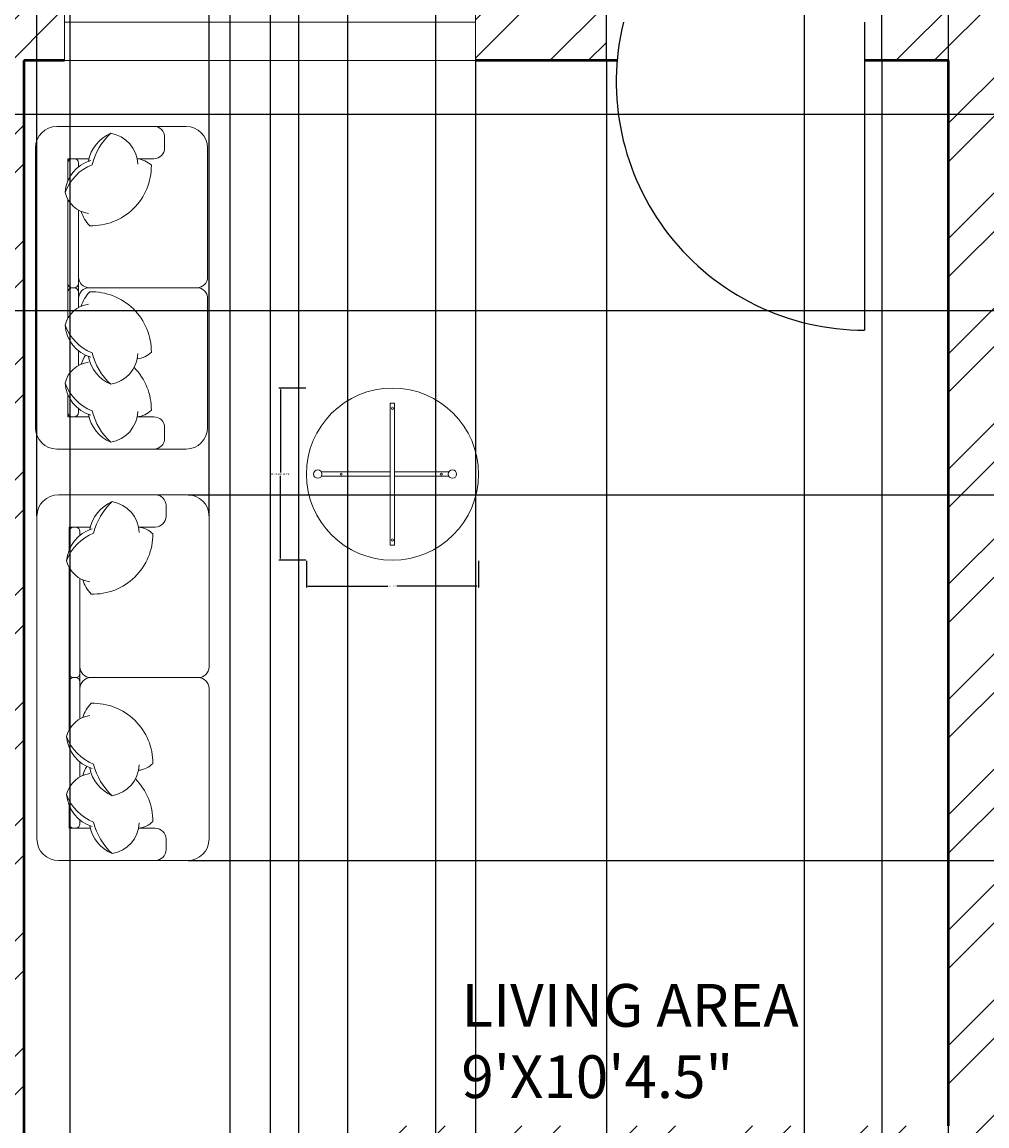
# Model space of a CAD drawing. Units: inches. Extents: x 1980 to 2738, y 1471 to 2568.
# Tile 9 of 22: x 2250 to 2363, y 1878 to 2007. Entities that reach past the tile are written whole.
import ezdxf

# ---------------------------------------------------------------- set-up
doc = ezdxf.new("R2010")
doc.units = ezdxf.units.IN
for name, color, linetype, lineweight in [('A-ANNO-DIMS', 2, 'Continuous', 18), ('A-AREA-IDEN', 7, 'Continuous', 18), ('A-DOOR', 31, 'Continuous', 25), ('A-FURN', 8, 'Continuous', 18), ('A-GLAZ', 141, 'Continuous', 18), ('A-WALL', 7, 'Continuous', 50)]:
    doc.layers.add(name, color=color, linetype=linetype, lineweight=lineweight)
doc.layers.add('A-WALL-PATT', color=9, linetype='Continuous', lineweight=13, true_color=0xd19cc7)
doc.styles.get("Standard").update_dxf_attribs({"font": 'arial.ttf'})
doc.dimstyles.get("Standard").update_dxf_attribs({"dimtxt": 0.18, "dimasz": 0.18, "dimexe": 0.18, "dimexo": 0.0625, "dimgap": 0.09, "dimtad": 0, "dimtih": 1, "dimtoh": 1, "dimdec": 4, "dimzin": 0, "dimdsep": 46, "dimtxsty": 'Standard', "dimcen": 0.09, "dimadec": 0, "dimazin": 0, "dimtfac": 1, "dimtdec": 4, "dimtofl": 0, "dimtmove": 0, "dimatfit": 3, "dimfxl": 1, "dimtolj": 1, "dimtzin": 0, "dimarcsym": 0})

# ---------------------------------------------------------------- blocks, each defined once
blk = doc.blocks.new('table r 343')
at = {"color": 0}
for p, q in [((-10, 10), (-10, 262.1)), ((10, 10), (10, 262.1)), ((-330.3, 10), (330.3, 10)), ((-330.3, 10), (-330.3, -10)), ((330.3, 10), (330.3, -10)), ((-330.3, -10), (330.3, -10)), ((-10, -330.3), (-10, -10)), ((10, -330.3), (10, -10))]:
    blk.add_line(p, q, dxfattribs=at)
for centre, radius in [((0, 0), 400), ((0, 278.7), 19.4), ((0, 226.8), 5), ((-306.1, 0), 5), ((306.1, 0), 5), ((0, -238.1), 5), ((0, -346.9), 19.4)]:
    blk.add_circle(centre, radius, dxfattribs=at)
blk = doc.blocks.new('WIN-48IN-WALL')
for p, q in [((0, 4.5), (0, 9)), ((0, 9), (0, 0)), ((48, 9), (0, 9)), ((48, 0), (48, 9)), ((48, 9), (48, 4.5)), ((48, 4.5), (0, 4.5)), ((0, 0), (48, 0))]:
    blk.add_line(p, q)
blk = doc.blocks.new('*D19')
at = {"layer": 'A-ANNO-DIMS', "color": 0, "lineweight": -2, "transparency": 16777216}
for p, q in [((2283.52, 1963.93), (2280.38, 1963.93)), ((2280.56, 1963.75), (2280.56, 1954.06)), ((2280.56, 1944), (2280.56, 1953.69)), ((2283.52, 1943.82), (2280.38, 1943.82))]:
    blk.add_line(p, q, dxfattribs=at)
at = {"layer": 'A-ANNO-DIMS', "color": 0, "transparency": 16777216}
for points in [[(2280.53, 1963.75), (2280.59, 1963.75), (2280.56, 1963.93)], [(2280.53, 1944), (2280.59, 1944), (2280.56, 1943.82)]]:
    blk.add_solid(points, dxfattribs=at)
at = {"layer": 'Defpoints', "color": 0, "transparency": 16777216}
for p in [(2283.58, 1963.93), (2280.56, 1943.82), (2283.58, 1943.82)]:
    blk.add_point(p, dxfattribs=at)
at = {"layer": 'A-ANNO-DIMS', "color": 0, "transparency": 16777216, "insert": (2280.56, 1953.88), "char_height": 0.18, "attachment_point": 5}
blk.add_mtext('\\A1;END TABLE 20 TYP.', dxfattribs=at)
blk = doc.blocks.new('*D20')
at = {"layer": 'A-ANNO-DIMS', "color": 0, "lineweight": -2, "transparency": 16777216}
for p, q in [((2283.58, 1943.76), (2283.58, 1940.62)), ((2303.69, 1943.76), (2303.69, 1940.62)), ((2283.76, 1940.8), (2293.1, 1940.8)), ((2303.51, 1940.8), (2294.16, 1940.8))]:
    blk.add_line(p, q, dxfattribs=at)
at = {"layer": 'A-ANNO-DIMS', "color": 0, "transparency": 16777216}
for points in [[(2283.76, 1940.83), (2283.76, 1940.77), (2283.58, 1940.8)], [(2303.51, 1940.83), (2303.51, 1940.77), (2303.69, 1940.8)]]:
    blk.add_solid(points, dxfattribs=at)
at = {"layer": 'Defpoints', "color": 0, "transparency": 16777216}
for p in [(2283.58, 1943.82), (2303.69, 1943.82), (2303.69, 1940.8)]:
    blk.add_point(p, dxfattribs=at)
at = {"layer": 'A-ANNO-DIMS', "color": 0, "transparency": 16777216, "insert": (2293.63, 1940.8), "char_height": 0.18, "attachment_point": 5}
blk.add_mtext('\\A1;20 TYP.', dxfattribs=at)
blk = doc.blocks.new('*D40')
at = {"layer": 'A-ANNO-DIMS', "color": 0, "lineweight": -2, "transparency": 16777216}
for p, q in [((2218.65, 2053.14), (2218.65, 1533.71)), ((2298.65, 2053.14), (2298.65, 1533.71)), ((2218.83, 1533.89), (2258.43, 1533.89)), ((2298.47, 1533.89), (2258.87, 1533.89))]:
    blk.add_line(p, q, dxfattribs=at)
at = {"layer": 'A-ANNO-DIMS', "color": 0, "transparency": 16777216}
for points in [[(2218.83, 1533.92), (2218.83, 1533.86), (2218.65, 1533.89)], [(2298.47, 1533.92), (2298.47, 1533.86), (2298.65, 1533.89)]]:
    blk.add_solid(points, dxfattribs=at)
at = {"layer": 'Defpoints', "color": 0, "transparency": 16777216}
for p in [(2218.65, 2053.21), (2298.65, 2053.21), (2298.65, 1533.89)]:
    blk.add_point(p, dxfattribs=at)
at = {"layer": 'A-ANNO-DIMS', "color": 0, "transparency": 16777216, "insert": (2258.65, 1533.89), "char_height": 0.18, "attachment_point": 5}
blk.add_mtext('\\A1;80', dxfattribs=at)
blk = doc.blocks.new('*D41')
at = {"layer": 'A-ANNO-DIMS', "color": 0, "lineweight": -2, "transparency": 16777216}
for p, q in [((2298.65, 2095.14), (2298.65, 1533.71)), ((2515.4, 2095.14), (2515.4, 1533.71)), ((2298.83, 1533.89), (2406.56, 1533.89)), ((2515.22, 1533.89), (2407.49, 1533.89))]:
    blk.add_line(p, q, dxfattribs=at)
at = {"layer": 'A-ANNO-DIMS', "color": 0, "transparency": 16777216}
for points in [[(2298.83, 1533.92), (2298.83, 1533.86), (2298.65, 1533.89)], [(2515.22, 1533.92), (2515.22, 1533.86), (2515.4, 1533.89)]]:
    blk.add_solid(points, dxfattribs=at)
at = {"layer": 'Defpoints', "color": 0, "transparency": 16777216}
for p in [(2298.65, 2095.21), (2515.4, 2095.21), (2515.4, 1533.89)]:
    blk.add_point(p, dxfattribs=at)
at = {"layer": 'A-ANNO-DIMS', "color": 0, "transparency": 16777216, "insert": (2407.03, 1533.89), "char_height": 0.18, "attachment_point": 5}
blk.add_mtext('\\A1;216.75', dxfattribs=at)
blk = doc.blocks.new('*D45')
at = {"layer": 'A-ANNO-DIMS', "color": 0, "lineweight": -2, "transparency": 16777216}
for p, q in [((2255.99, 1694.77), (2255.99, 2507.54)), ((2256.17, 2507.36), (2267.22, 2507.36)), ((2279.21, 2507.36), (2268.15, 2507.36)), ((2279.39, 1694.77), (2279.39, 2507.54))]:
    blk.add_line(p, q, dxfattribs=at)
at = {"layer": 'A-ANNO-DIMS', "color": 0, "transparency": 16777216}
for points in [[(2256.17, 2507.39), (2256.17, 2507.33), (2255.99, 2507.36)], [(2279.21, 2507.39), (2279.21, 2507.33), (2279.39, 2507.36)]]:
    blk.add_solid(points, dxfattribs=at)
at = {"layer": 'Defpoints', "color": 0, "transparency": 16777216}
for p in [(2279.39, 2507.36), (2255.99, 1694.71), (2279.39, 1694.71)]:
    blk.add_point(p, dxfattribs=at)
at = {"layer": 'A-ANNO-DIMS', "color": 0, "transparency": 16777216, "insert": (2267.69, 2507.36), "char_height": 0.18, "attachment_point": 5}
blk.add_mtext('\\A1;23.407', dxfattribs=at)
blk = doc.blocks.new('*D50')
at = {"layer": 'A-ANNO-DIMS', "color": 0, "lineweight": -2, "transparency": 16777216}
for p, q in [((2288.43, 1708.09), (2288.43, 2507.54)), ((2288.61, 2507.36), (2314.71, 2507.36)), ((2341.6, 2507.36), (2315.5, 2507.36)), ((2341.78, 1708.09), (2341.78, 2507.54))]:
    blk.add_line(p, q, dxfattribs=at)
at = {"layer": 'A-ANNO-DIMS', "color": 0, "transparency": 16777216}
for points in [[(2288.61, 2507.39), (2288.61, 2507.33), (2288.43, 2507.36)], [(2341.6, 2507.39), (2341.6, 2507.33), (2341.78, 2507.36)]]:
    blk.add_solid(points, dxfattribs=at)
at = {"layer": 'Defpoints', "color": 0, "transparency": 16777216}
for p in [(2341.78, 2507.36), (2288.43, 1708.03), (2341.78, 1708.03)]:
    blk.add_point(p, dxfattribs=at)
at = {"layer": 'A-ANNO-DIMS', "color": 0, "transparency": 16777216, "insert": (2315.11, 2507.36), "char_height": 0.18, "attachment_point": 5}
blk.add_mtext('\\A1;53.34', dxfattribs=at)
blk = doc.blocks.new('*D51')
at = {"layer": 'A-ANNO-DIMS', "color": 0, "lineweight": -2, "transparency": 16777216}
for p, q in [((2341.78, 1708.09), (2341.78, 2507.54)), ((2341.96, 2507.36), (2349.72, 2507.36)), ((2358.4, 2507.36), (2350.63, 2507.36)), ((2358.58, 1694.77), (2358.58, 2507.54))]:
    blk.add_line(p, q, dxfattribs=at)
at = {"layer": 'A-ANNO-DIMS', "color": 0, "transparency": 16777216}
for points in [[(2341.96, 2507.39), (2341.96, 2507.33), (2341.78, 2507.36)], [(2358.4, 2507.39), (2358.4, 2507.33), (2358.58, 2507.36)]]:
    blk.add_solid(points, dxfattribs=at)
at = {"layer": 'Defpoints', "color": 0, "transparency": 16777216}
for p in [(2358.58, 2507.36), (2341.78, 1708.03), (2358.58, 1694.71)]:
    blk.add_point(p, dxfattribs=at)
at = {"layer": 'A-ANNO-DIMS', "color": 0, "transparency": 16777216, "insert": (2350.18, 2507.36), "char_height": 0.18, "attachment_point": 5}
blk.add_mtext('\\A1;16.807', dxfattribs=at)
blk = doc.blocks.new('*D53')
at = {"layer": 'A-ANNO-DIMS', "color": 0, "lineweight": -2, "transparency": 16777216}
for p, q in [((2318.63, 2002.14), (2318.63, 1533.71)), ((2350.79, 2002.14), (2350.79, 1533.71)), ((2318.81, 1533.89), (2334.25, 1533.89)), ((2350.61, 1533.89), (2335.18, 1533.89))]:
    blk.add_line(p, q, dxfattribs=at)
at = {"layer": 'A-ANNO-DIMS', "color": 0, "transparency": 16777216}
for points in [[(2318.81, 1533.92), (2318.81, 1533.86), (2318.63, 1533.89)], [(2350.61, 1533.92), (2350.61, 1533.86), (2350.79, 1533.89)]]:
    blk.add_solid(points, dxfattribs=at)
at = {"layer": 'Defpoints', "color": 0, "transparency": 16777216}
for p in [(2318.63, 2002.21), (2350.79, 2002.21), (2350.79, 1533.89)]:
    blk.add_point(p, dxfattribs=at)
at = {"layer": 'A-ANNO-DIMS', "color": 0, "transparency": 16777216, "insert": (2334.71, 1533.89), "char_height": 0.18, "attachment_point": 5}
blk.add_mtext('\\A1;32.155', dxfattribs=at)
blk = doc.blocks.new('*D54')
at = {"layer": 'A-ANNO-DIMS', "color": 0, "lineweight": -2, "transparency": 16777216}
for p, q in [((2252.1, 1949.01), (2252.1, 2507.54)), ((2252.28, 2507.36), (2261.78, 2507.36)), ((2272.03, 2507.36), (2262.53, 2507.36)), ((2272.21, 1949.01), (2272.21, 2507.54))]:
    blk.add_line(p, q, dxfattribs=at)
at = {"layer": 'A-ANNO-DIMS', "color": 0, "transparency": 16777216}
for points in [[(2252.28, 2507.39), (2252.28, 2507.33), (2252.1, 2507.36)], [(2272.03, 2507.39), (2272.03, 2507.33), (2272.21, 2507.36)]]:
    blk.add_solid(points, dxfattribs=at)
at = {"layer": 'Defpoints', "color": 0, "transparency": 16777216}
for p in [(2272.21, 2507.36), (2252.1, 1948.95), (2272.21, 1948.95)]:
    blk.add_point(p, dxfattribs=at)
at = {"layer": 'A-ANNO-DIMS', "color": 0, "transparency": 16777216, "insert": (2262.16, 2507.36), "char_height": 0.18, "attachment_point": 5}
blk.add_mtext('\\A1;20.11', dxfattribs=at)
blk = doc.blocks.new('*D55')
at = {"layer": 'A-ANNO-DIMS', "color": 0, "lineweight": -2, "transparency": 16777216}
for p, q in [((2269.76, 1951.46), (2689.91, 1951.46)), ((2689.73, 1951.28), (2689.73, 1930.28)), ((2689.73, 1908.91), (2689.73, 1929.91)), ((2269.76, 1908.73), (2689.91, 1908.73))]:
    blk.add_line(p, q, dxfattribs=at)
at = {"layer": 'A-ANNO-DIMS', "color": 0, "transparency": 16777216}
for points in [[(2689.7, 1951.28), (2689.76, 1951.28), (2689.73, 1951.46)], [(2689.7, 1908.91), (2689.76, 1908.91), (2689.73, 1908.73)]]:
    blk.add_solid(points, dxfattribs=at)
at = {"layer": 'Defpoints', "color": 0, "transparency": 16777216}
for p in [(2269.7, 1951.46), (2689.73, 1951.46), (2269.7, 1908.73)]:
    blk.add_point(p, dxfattribs=at)
at = {"layer": 'A-ANNO-DIMS', "color": 0, "transparency": 16777216, "insert": (2689.73, 1930.09), "char_height": 0.18, "attachment_point": 5}
blk.add_mtext('\\A1;42.735', dxfattribs=at)
blk = doc.blocks.new('*D56')
at = {"layer": 'A-ANNO-DIMS', "color": 0, "lineweight": -2, "transparency": 16777216}
for p, q in [((2114.15, 1995.93), (2689.91, 1995.93)), ((2689.73, 1995.75), (2689.73, 1984.65)), ((2689.73, 1973.18), (2689.73, 1984.28)), ((2114.15, 1973), (2689.91, 1973))]:
    blk.add_line(p, q, dxfattribs=at)
at = {"layer": 'A-ANNO-DIMS', "color": 0, "transparency": 16777216}
for points in [[(2689.7, 1995.75), (2689.76, 1995.75), (2689.73, 1995.93)], [(2689.7, 1973.18), (2689.76, 1973.18), (2689.73, 1973)]]:
    blk.add_solid(points, dxfattribs=at)
at = {"layer": 'Defpoints', "color": 0, "transparency": 16777216}
for p in [(2114.08, 1995.93), (2689.73, 1995.93), (2114.08, 1973)]:
    blk.add_point(p, dxfattribs=at)
at = {"layer": 'A-ANNO-DIMS', "color": 0, "transparency": 16777216, "insert": (2689.73, 1984.47), "char_height": 0.18, "attachment_point": 5}
blk.add_mtext('\\A1;22.935', dxfattribs=at)
blk = doc.blocks.new('*D64')
at = {"layer": 'A-ANNO-DIMS', "color": 0, "lineweight": -2, "transparency": 16777216}
for p, q in [((2303.33, 2002.14), (2303.33, 1533.71)), ((2318.63, 2002.14), (2318.63, 1533.71)), ((2303.51, 1533.89), (2310.67, 1533.89)), ((2318.45, 1533.89), (2311.3, 1533.89))]:
    blk.add_line(p, q, dxfattribs=at)
at = {"layer": 'A-ANNO-DIMS', "color": 0, "transparency": 16777216}
for points in [[(2303.51, 1533.92), (2303.51, 1533.86), (2303.33, 1533.89)], [(2318.45, 1533.92), (2318.45, 1533.86), (2318.63, 1533.89)]]:
    blk.add_solid(points, dxfattribs=at)
at = {"layer": 'Defpoints', "color": 0, "transparency": 16777216}
for p in [(2303.33, 2002.21), (2318.63, 2002.21), (2318.63, 1533.89)]:
    blk.add_point(p, dxfattribs=at)
at = {"layer": 'A-ANNO-DIMS', "color": 0, "transparency": 16777216, "insert": (2310.98, 1533.89), "char_height": 0.18, "attachment_point": 5}
blk.add_mtext('\\A1;15.3', dxfattribs=at)
blk = doc.blocks.new('*D66')
at = {"layer": 'A-ANNO-DIMS', "color": 0, "lineweight": -2, "transparency": 16777216}
for p, q in [((2274.65, 2095.14), (2274.65, 1533.71)), ((2282.65, 2095.14), (2282.65, 1533.71)), ((2274.83, 1533.89), (2278.5, 1533.89)), ((2282.47, 1533.89), (2278.8, 1533.89))]:
    blk.add_line(p, q, dxfattribs=at)
at = {"layer": 'A-ANNO-DIMS', "color": 0, "transparency": 16777216}
for points in [[(2274.83, 1533.92), (2274.83, 1533.86), (2274.65, 1533.89)], [(2282.47, 1533.92), (2282.47, 1533.86), (2282.65, 1533.89)]]:
    blk.add_solid(points, dxfattribs=at)
at = {"layer": 'Defpoints', "color": 0, "transparency": 16777216}
for p in [(2274.65, 2095.21), (2282.65, 2095.21), (2282.65, 1533.89)]:
    blk.add_point(p, dxfattribs=at)
at = {"layer": 'A-ANNO-DIMS', "color": 0, "transparency": 16777216, "insert": (2278.65, 1533.89), "char_height": 0.18, "attachment_point": 5}
blk.add_mtext('\\A1;8', dxfattribs=at)

msp = doc.modelspace()

# ---------------------------------------------------------------- hatches: boundary and pattern name
at = {"layer": 'A-WALL-PATT'}
h = msp.add_hatch(dxfattribs=at)
h.set_pattern_fill('ANSI32', color=256)
h.paths.add_polyline_path([(2257.5661, 2416.2064), (2257.5661, 2420.7064), (2250.5833, 2420.7064), (2250.5833, 2462.7064), (2246.0833, 2462.7064), (2246.0833, 2420.7064), (2237.0791, 2420.7064), (2237.0791, 2411.7064), (2246.0833, 2411.7064), (2246.0833, 2291.7064), (2242.6109, 2291.7064), (2242.6109, 2287.2064), (2246.0833, 2287.2064), (2250.5833, 2287.2064), (2250.5833, 2291.7064), (2250.5833, 2411.7064), (2257.5661, 2411.7064)])
h.paths.add_polyline_path([(2387.0396, 2416.2064), (2387.0396, 2420.7064), (2367.5833, 2420.7064), (2367.5833, 2462.7064), (2358.5833, 2462.7064), (2358.5833, 2420.7064), (2329.3087, 2420.7064), (2329.3087, 2411.7064), (2358.5833, 2411.7064), (2358.5833, 2321.7275), (2358.5833, 2309.7064), (2347.3089, 2309.7064), (2293.3089, 2309.7064), (2293.3089, 2259.0771), (2297.8089, 2259.0771), (2297.8089, 2305.2064), (2347.3089, 2305.2064), (2347.3089, 2284.7412), (2351.8089, 2284.7412), (2351.8089, 2305.2064), (2372.3188, 2305.2064), (2372.3761, 2284.3899), (2377.0295, 2284.3899), (2377.0295, 2299.3058), (2377.0295, 2305.2064), (2426.5295, 2305.2064), (2426.5295, 2257.5573), (2431.0295, 2257.5573), (2431.0295, 2309.7064), (2377.0295, 2309.7064), (2367.5833, 2309.7064), (2367.5833, 2321.7275), (2367.5833, 2411.7064), (2387.0396, 2411.7064)])
h.paths.add_polyline_path([(2448.5267, 2416.2064), (2448.5267, 2420.7064), (2423.0396, 2420.7064), (2423.0396, 2411.7064), (2448.5267, 2411.7064)])
h.paths.add_polyline_path([(2130.9128, 2416.2064), (2130.9128, 2420.7064), (2105.0833, 2420.7064), (2105.0833, 2386.6942), (2114.0833, 2386.6942), (2114.0833, 2411.7064), (2130.9128, 2411.7064)])
h.paths.add_polyline_path([(2212.9478, 2420.7064), (2190.9128, 2420.7064), (2190.9128, 2411.7064), (2212.9478, 2411.7064), (2212.9478, 2416.2064)])
h.paths.add_polyline_path([(2114.0833, 2326.6942), (2105.0833, 2326.6942), (2105.0833, 2291.7064), (2081.0833, 2291.7064), (2081.0833, 2287.2064), (2105.0833, 2287.2064), (2105.0833, 2276.1935), (2114.0833, 2276.1935), (2114.0833, 2287.2064), (2166.3825, 2287.2064), (2166.3825, 2289.4564), (2166.3825, 2291.7064), (2114.0833, 2291.7064)])
h.paths.add_polyline_path([(2114.0833, 2252.1935), (2105.0833, 2252.1935), (2105.0833, 2233.2064), (2081.0833, 2233.2064), (2081.0833, 2228.7064), (2105.0833, 2228.7064), (2105.0833, 2213.4478), (2114.0833, 2213.4478), (2114.0833, 2228.7064), (2195.0833, 2228.7064), (2199.5833, 2228.7064), (2208.4455, 2228.7064), (2208.4455, 2230.9564), (2208.4455, 2233.2064), (2199.5833, 2233.2064), (2199.5833, 2287.2064), (2206.8904, 2287.2064), (2206.8904, 2289.4564), (2206.8904, 2291.7064), (2189.446, 2291.7064), (2189.446, 2289.4564), (2189.446, 2287.2064), (2195.0833, 2287.2064), (2195.0833, 2233.2064), (2114.0833, 2233.2064)])
h.paths.add_polyline_path([(2114.0833, 2153.4478), (2109.5833, 2153.4478), (2105.0833, 2153.4478), (2105.0833, 2135.2374), (2114.0833, 2135.2374)], flags=17)
h.paths.add_polyline_path([(2135.9619, 2095.4081), (2140.1805, 2095.4081), (2140.1805, 2104.2064), (2114.0833, 2104.2064), (2114.0833, 2110.3997), (2109.5833, 2110.3997), (2105.0833, 2110.3997), (2105.0833, 2104.2064), (2081.0833, 2104.2064), (2081.0833, 2099.7064), (2105.0833, 2099.7064), (2127.5416, 2099.8532), (2127.5416, 2056.9393), (2136.2133, 2056.9393)], flags=17)
h.paths.add_polyline_path([(2255.4895, 2104.2064), (2250.5833, 2104.2064), (2250.5833, 2233.2064), (2246.0833, 2233.2064), (2242.4941, 2233.2064), (2242.4941, 2228.7064), (2246.0833, 2228.7064), (2246.0833, 2104.2064), (2163.6825, 2104.2064), (2163.6825, 2099.8072), (2163.6825, 2095.4081), (2191.4325, 2095.4081), (2191.4325, 2011.2064), (2186.0833, 2011.2064), (2136.5143, 2010.8824), (2136.3702, 2032.9403), (2131.9559, 2032.9115), (2127.5416, 2032.8826), (2127.5416, 2006.7064), (2105.0833, 2006.7064), (2081.0833, 2006.7064), (2081.0833, 2002.2064), (2105.0833, 2002.2064), (2105.0833, 1995.9329), (2114.0833, 1995.9329), (2114.0833, 2002.2064), (2246.0833, 2002.2064), (2246.0833, 1877.7064), (2242.1358, 1877.7064), (2242.1358, 1873.2064), (2250.5833, 1873.2064), (2250.5833, 2002.2064), (2255.3335, 2002.2064), (2255.3335, 2011.2064), (2195.9325, 2011.2064), (2195.9325, 2095.2064), (2255.4895, 2095.2064), (2255.4895, 2099.5471)])
h.paths.add_polyline_path([(2199.5833, 1873.2064), (2209.827, 1873.2064), (2209.827, 1875.4564), (2209.827, 1877.7064), (2114.0833, 1877.7064), (2114.0833, 1890.0968), (2105.0833, 1890.0968), (2105.0833, 1877.7064), (2081.0833, 1877.7064), (2081.0833, 1873.2064), (2105.0833, 1873.2064), (2105.0833, 1857.7279), (2114.0833, 1857.7279), (2114.0833, 1873.2064), (2195.0833, 1873.2064), (2195.0833, 1819.2064), (2190.298, 1819.2064), (2190.298, 1814.7064), (2209.8976, 1814.7064), (2209.8976, 1816.9564), (2209.8976, 1819.2064), (2199.5833, 1819.2064)])
h.paths.add_polyline_path([(2114.0833, 1814.7064), (2166.2538, 1814.7064), (2166.2538, 1816.9564), (2166.2538, 1819.2064), (2114.0833, 1819.2064), (2114.0833, 1833.7279), (2109.5833, 1833.7279), (2105.0833, 1833.7279), (2105.0833, 1819.2064), (2081.0833, 1819.2064), (2081.0833, 1814.7064), (2105.0833, 1814.7064), (2105.0833, 1782.5516), (2114.0833, 1782.5516)])
h.paths.add_polyline_path([(2114.0833, 1722.5516), (2109.5833, 1722.5516), (2105.0833, 1722.5516), (2105.0833, 1685.7064), (2124.5104, 1685.7064), (2124.5104, 1690.2064), (2124.5104, 1694.7064), (2114.0833, 1694.7064)])
h.paths.add_polyline_path([(2218.8787, 1694.7064), (2184.5104, 1694.7064), (2184.5104, 1685.7064), (2218.8787, 1685.7064), (2218.8787, 1690.2064)])
h.paths.add_polyline_path([(2250.5833, 1819.2064), (2242.6431, 1819.2064), (2242.6431, 1816.9564), (2242.6431, 1814.7064), (2246.0833, 1814.7064), (2246.0833, 1694.7064), (2240.4035, 1694.7064), (2240.4035, 1690.2064), (2240.4035, 1685.7064), (2246.0833, 1685.7064), (2246.0833, 1643.7064), (2250.5833, 1643.7064), (2250.5833, 1685.7064), (2255.9859, 1685.7064), (2255.9859, 1690.2064), (2255.9859, 1694.7064), (2250.5833, 1694.7064)])
h.paths.add_polyline_path([(2297.4764, 1694.7064), (2279.3934, 1694.7064), (2279.3934, 1690.2064), (2279.3934, 1685.7064), (2297.4764, 1685.7064), (2297.4764, 1690.2064)])
h.paths.add_polyline_path([(2377.1596, 1694.7064), (2367.5833, 1694.7064), (2367.5833, 1787.7064), (2431.0295, 1787.7064), (2431.0295, 1792.2064), (2431.0295, 1849.4149), (2428.7795, 1849.4149), (2426.5295, 1849.4149), (2426.5295, 1792.2064), (2421.5833, 1792.2064), (2367.5833, 1792.2064), (2297.8089, 1792.2064), (2297.8089, 1850.2946), (2295.5589, 1850.2946), (2293.3089, 1850.2946), (2293.3089, 1792.2064), (2293.3089, 1787.7064), (2297.8089, 1787.7064), (2358.5833, 1787.7064), (2358.5833, 1694.7064), (2333.4764, 1694.7064), (2333.4764, 1685.7064), (2358.5833, 1685.7064), (2358.5833, 1643.7064), (2367.5833, 1643.7064), (2367.5833, 1685.7064), (2377.1596, 1685.7064)])
h.paths.add_polyline_path([(2442.4912, 1694.7064), (2413.1596, 1694.7064), (2413.1596, 1685.7064), (2442.4912, 1685.7064)])
h.paths.add_polyline_path([(2480.0833, 1814.7064), (2483.4816, 1814.7064), (2483.4816, 1817.9384), (2483.4816, 1819.2064), (2475.5833, 1819.2064), (2475.5833, 1694.7064), (2470.7283, 1694.7064), (2470.7283, 1685.7064), (2475.5833, 1685.7064), (2475.5833, 1643.7064), (2480.0833, 1643.7064), (2480.0833, 1685.7064), (2486.3293, 1685.7064), (2486.3293, 1690.2064), (2486.3293, 1694.7064), (2480.0833, 1694.7064)])
h.paths.add_polyline_path([(2621.0833, 1721.7349), (2612.0833, 1721.7349), (2612.0833, 1694.7064), (2586.1453, 1694.7064), (2586.1453, 1685.7064), (2621.0833, 1685.7064)])
h.paths.add_polyline_path([(2526.1453, 1690.2064), (2526.1453, 1694.7064), (2511.584, 1694.7064), (2511.584, 1690.2064), (2511.584, 1685.7064), (2526.1453, 1685.7064)])
h.paths.add_polyline_path([(2645.0833, 1819.2064), (2621.0833, 1819.2064), (2621.0833, 1835.8527), (2616.5833, 1835.8527), (2612.0833, 1835.8527), (2612.0833, 1819.2064), (2560.2541, 1819.2064), (2560.2541, 1814.7064), (2612.0833, 1814.7064), (2612.0833, 1781.7349), (2621.0833, 1781.7349), (2621.0833, 1814.7064), (2645.0833, 1814.7064)])
h.paths.add_polyline_path([(2645.0833, 1877.7064), (2621.0833, 1877.7064), (2621.0833, 1886.4375), (2612.0833, 1886.4375), (2612.0833, 1877.7064), (2517.1032, 1877.7064), (2517.1032, 1875.4564), (2517.1032, 1873.2064), (2526.5833, 1873.2064), (2526.5833, 1819.2064), (2516.6454, 1819.2064), (2516.6454, 1816.9564), (2516.6454, 1814.7064), (2536.4445, 1814.7064), (2536.4445, 1816.9564), (2536.4445, 1819.2064), (2531.0833, 1819.2064), (2531.0833, 1873.2064), (2612.0833, 1873.2064), (2612.0833, 1859.8527), (2621.0833, 1859.8527), (2621.0833, 1873.2064), (2645.0833, 1873.2064)])
h.paths.add_polyline_path([(2645.0833, 2006.7064), (2621.0833, 2006.7064), (2588.5085, 2006.7064), (2588.5085, 2052.9125), (2579.9045, 2052.9125), (2579.9045, 2011.2064), (2519.9045, 2011.2064), (2519.9045, 2095.2064), (2553.1204, 2095.2064), (2553.1204, 2104.2064), (2480.0833, 2104.2064), (2480.0833, 2228.7064), (2484.3832, 2228.7064), (2484.3832, 2230.9564), (2484.3832, 2233.2064), (2475.5833, 2233.2064), (2475.5833, 2104.2064), (2463.1308, 2104.2064), (2463.1308, 2095.2064), (2501.2463, 2095.2064), (2510.9045, 2095.2064), (2515.4045, 2095.2064), (2515.4045, 2011.2064), (2510.9045, 2011.2064), (2501.2463, 2011.2064), (2462.5957, 2011.2064), (2462.5957, 2002.2064), (2475.5833, 2002.2064), (2475.5833, 1873.2064), (2483.6146, 1873.2064), (2483.6146, 1875.4564), (2483.6146, 1877.7064), (2480.0833, 1877.7064), (2480.0833, 2002.2064), (2612.0833, 2002.2064), (2612.0833, 1996.309), (2621.0833, 1996.309), (2621.0833, 2002.2064), (2645.0833, 2002.2064)])
h.paths.add_polyline_path([(2588.5085, 2099.7277), (2621.0833, 2099.7277), (2645.0833, 2099.7064), (2645.0833, 2104.2064), (2621.0833, 2104.2064), (2621.0833, 2109.0038), (2616.5833, 2109.0038), (2612.0833, 2109.0038), (2612.0833, 2104.2064), (2575.0621, 2104.2064), (2575.0621, 2099.7064), (2575.0621, 2095.2064), (2579.9045, 2095.2064), (2579.9045, 2076.9125), (2588.5085, 2076.9125)], flags=17)
h.paths.add_polyline_path([(2367.5833, 2002.2064), (2373.7228, 2002.2064), (2373.7228, 2006.7064), (2373.7228, 2011.2064), (2350.7889, 2011.2064), (2350.7889, 2006.7064), (2350.7889, 2002.2064), (2358.5833, 2002.2064), (2358.5833, 1877.7064), (2293.3089, 1877.7064), (2293.3089, 1870.4987), (2297.8089, 1870.4987), (2297.8089, 1873.2064), (2347.3089, 1873.2064), (2347.3089, 1847.2208), (2351.8089, 1847.2208), (2351.8089, 1873.2064), (2372.5295, 1873.2064), (2372.5295, 1847.8619), (2377.0295, 1847.8619), (2377.0295, 1873.2064), (2426.5295, 1873.2064), (2426.5295, 1868.7339), (2431.0295, 1868.7339), (2431.0295, 1877.7064), (2367.5833, 1877.7064)])
h.paths.add_polyline_path([(2531.0833, 2287.2064), (2534.2285, 2287.2064), (2534.2285, 2291.7064), (2516.7886, 2291.7064), (2516.7886, 2287.2064), (2526.5833, 2287.2064), (2526.5833, 2233.2064), (2517.9112, 2233.2064), (2517.9112, 2230.9564), (2517.9112, 2228.7064), (2526.5833, 2228.7064), (2531.0833, 2228.7064), (2612.0833, 2228.7064), (2612.0833, 2206.8504), (2621.0833, 2206.8504), (2621.0833, 2228.7064), (2645.0833, 2228.7064), (2645.0833, 2233.2064), (2621.0833, 2233.2064), (2621.0833, 2241.8536), (2616.5833, 2241.8536), (2612.0833, 2241.8536), (2612.0833, 2233.2064), (2531.0833, 2233.2064)])
h.paths.add_polyline_path([(2645.0833, 2291.7064), (2621.0833, 2291.7064), (2621.0833, 2323.0138), (2616.5833, 2323.0138), (2612.0833, 2323.0138), (2612.0833, 2291.7064), (2559.6852, 2291.7064), (2559.6852, 2289.4564), (2559.6852, 2287.2064), (2612.0833, 2287.2064), (2612.0833, 2265.8536), (2621.0833, 2265.8536), (2621.0833, 2287.2064), (2645.0833, 2287.2064)])
h.paths.add_polyline_path([(2621.0833, 2420.7064), (2582.8189, 2420.7064), (2582.8189, 2411.7064), (2612.0833, 2411.7064), (2612.0833, 2383.0138), (2621.0833, 2383.0138)])
h.paths.add_polyline_path([(2480.0833, 2411.7064), (2485.7342, 2411.7064), (2485.7342, 2416.2064), (2485.7342, 2420.7064), (2480.0833, 2420.7064), (2480.0833, 2462.7064), (2475.5833, 2462.7064), (2475.5833, 2420.7064), (2469.4083, 2420.7064), (2469.4083, 2411.7064), (2475.5833, 2411.7064), (2475.5833, 2291.7064), (2475.5833, 2287.2064), (2482.9195, 2287.2064), (2482.9195, 2289.4564), (2482.9195, 2291.7064), (2480.0833, 2291.7064)])
h.paths.add_polyline_path([(2367.5833, 2228.7064), (2431.0295, 2228.7064), (2431.0295, 2233.2064), (2431.0295, 2237.4203), (2428.7795, 2237.4203), (2426.5295, 2237.4203), (2426.5295, 2233.2064), (2377.0295, 2233.2064), (2377.0295, 2260.3837), (2372.4423, 2260.3837), (2372.517, 2233.2635), (2351.8089, 2233.2064), (2351.8089, 2260.7412), (2347.3089, 2260.7412), (2347.3089, 2233.2064), (2297.8089, 2233.2064), (2297.8089, 2236.9324), (2293.3089, 2236.9324), (2293.3089, 2228.7064), (2358.5833, 2228.7064), (2358.5833, 2104.2064), (2353.3665, 2104.2064), (2353.3665, 2095.2064), (2373.8869, 2095.2064), (2373.8869, 2099.7064), (2373.8869, 2104.2064), (2367.5833, 2104.2064)])
h.paths.add_polyline_path([(2321.2323, 2104.2064), (2303.4895, 2104.2064), (2303.4895, 2095.2064), (2321.2323, 2095.2064), (2321.2323, 2099.7064)], flags=0)
h.paths.add_polyline_path([(2415.1308, 2099.7064), (2415.1308, 2104.2064), (2404.81, 2104.2064), (2404.81, 2095.2064), (2415.1308, 2095.2064)], flags=17)
h.paths.add_polyline_path([(2318.6336, 2011.2064), (2303.3335, 2011.2064), (2303.3335, 2002.2064), (2318.6336, 2002.2064)], flags=0)
h.paths.add_polyline_path([(2414.5957, 2011.2064), (2406.2461, 2011.2064), (2406.2461, 2006.7064), (2406.2461, 2002.2064), (2414.5957, 2002.2064)], flags=17)
h = msp.add_hatch(dxfattribs=at)
h.set_pattern_fill('ANSI32', color=256)
h.paths.add_polyline_path([(2321.2323, 2104.2064), (2303.4895, 2104.2064), (2303.4895, 2095.2064), (2321.2323, 2095.2064), (2321.2323, 2099.7064)])
h.paths.add_polyline_path([(2318.6336, 2011.2064), (2303.3335, 2011.2064), (2303.3335, 2002.2064), (2318.6336, 2002.2064)])
h.paths.add_polyline_path([(2114.0833, 1972.9983), (2109.5833, 1972.9983), (2105.0833, 1972.9983), (2105.0833, 1950.0968), (2114.0833, 1950.0968)])
h.paths.add_polyline_path([(2621.0833, 1971.9446), (2616.5833, 1971.9446), (2612.0833, 1971.9446), (2612.0833, 1946.4375), (2621.0833, 1946.4375)])
h.paths.add_polyline_path([(2621.0833, 2146.8504), (2612.0833, 2146.8504), (2612.0833, 2134.6713), (2621.0833, 2134.6713)])

# ---------------------------------------------------------------- linework, layer by layer
at = {"layer": 'A-DOOR'}
for p, q in [((2318.6336, 2002.2064), (2318.6336, 2011.2064)), ((2350.7889, 2002.2064), (2350.7889, 2011.2064)), ((2348.7889, 2006.7064), (2348.7889, 1970.7064))]:
    msp.add_line(p, q, dxfattribs=at)
msp.add_arc((2348.7889, 1999.7164), 29.01, 166.057272, 270, dxfattribs=at)
at = {"layer": 'A-FURN', "ltscale": 0.03}
for points in [[(2272.0418, 1976.9142, -0.41421356), (2270.7848, 1975.6573, -0.41421356), (2272.0418, 1974.4004), (2272.0418, 1959.3174, -0.41421356), (2269.5279, 1956.8035), (2254.4449, 1956.8035, -0.41421356), (2251.9311, 1959.3174), (2251.9311, 1991.9972, -0.41421356), (2254.4449, 1994.5111), (2269.5279, 1994.5111, -0.41421356), (2272.0418, 1991.9972), (2272.0418, 1976.9142, -0.41421356), (2270.7848, 1975.6573, -0.41421356), (2272.0418, 1974.4004)], [(2272.2106, 1931.3503, -0.41421356), (2270.9537, 1930.0934, -0.41421356), (2272.2106, 1928.8365), (2272.2106, 1911.2397, -0.41421356), (2269.6968, 1908.7258), (2254.6138, 1908.7258, -0.41421356), (2252.1, 1911.2397), (2252.1, 1948.9472, -0.41421356), (2254.6138, 1951.461), (2269.6968, 1951.461, -0.41421356), (2272.2106, 1948.9472), (2272.2106, 1931.3503, -0.41421356), (2270.9537, 1930.0934, -0.41421356), (2272.2106, 1928.8365)]]:
    msp.add_lwpolyline(points, format="xyb", dxfattribs=at)
at = {"layer": 'A-FURN'}
for points in [[(2265.7572, 1994.5111, -0.41421356), (2267.0141, 1993.2541), (2267.0141, 1991.9972, -0.41421356), (2265.7572, 1990.7403), (2263.8098, 1990.7403)], [(2260.7176, 1993.7111, 0.14772988), (2258.5575, 1990.0375, 0.21334276), (2255.3893, 1986.7961, 0.17866181)], [(2263.8858, 1990.1095, 0.35677236), (2260.7176, 1993.7111, 0.24954205), (2258.1068, 1990.4478, -9.61688035)], [(2258.3853, 1990.545, 0.30666349), (2255.3893, 1986.7961, 0.30632997), (2258.1255, 1984.347, -0.87284716)], [(2256.9588, 1989.7811), (2256.9588, 1990.2375, 0.41421356), (2256.456, 1990.7403), (2256.2046, 1990.7403, 0.41421356), (2255.7018, 1990.2375)], [(2263.8092, 1990.743, -0.16554063), (2265.4699, 1989.9655, -0.42598917), (2258.2695, 1982.9064, -0.12152332), (2257.277, 1984.5821, 7.11546429)], [(2255.7018, 1986.0051), (2255.7018, 1976.1601, 0.41421356), (2256.2046, 1975.6573), (2256.456, 1975.6573, 0.41421356), (2256.9588, 1976.1601), (2256.9588, 1984.7394, 0.41421356)], [(2256.9588, 1976.9142, 0.41421356), (2258.2157, 1975.6573)], [(2256.9588, 1976.9142, 0.41421356), (2258.2157, 1975.6573), (2270.7848, 1975.6573, 0.41421356)], [(2255.7018, 1972.0805), (2255.7018, 1975.1545, -0.41421356), (2256.2046, 1975.6573), (2256.456, 1975.6573, -0.41421356), (2256.9588, 1975.1545), (2256.9588, 1973.3462, -0.41421356)], [(2256.9588, 1974.4004, -0.41421356), (2258.2157, 1975.6573)], [(2256.9588, 1974.4004, -0.41421356), (2258.2157, 1975.6573), (2270.7848, 1975.6573, -0.41421356)], [(2263.8092, 1967.3425, 0.16554063), (2265.4699, 1968.1201, 0.42598917), (2258.2695, 1975.1792, 0.12152332), (2257.277, 1973.5035, -7.11546429)], [(2258.3853, 1967.5406, -0.30666349), (2255.3893, 1971.2895, -0.30632997), (2258.1255, 1973.7386, 0.87284716)], [(2260.7176, 1964.3745, -0.14772988), (2258.5575, 1968.0481, -0.21334276), (2255.3893, 1971.2895, -0.17866181)], [(2256.9588, 1968.3044), (2256.9588, 1966.5752, -0.41421356)], [(2257.7684, 1967.7863, 0.07186538), (2257.277, 1966.7325, -7.11546429)], [(2263.8858, 1967.976, -0.35677236), (2260.7176, 1964.3745, -0.24954205), (2258.1068, 1967.6378, 9.61688035)], [(2258.3853, 1960.7696, -0.30666349), (2255.3893, 1964.5185, -0.30632997), (2258.1255, 1966.9676, 0.87284716)], [(2263.8092, 1960.5716, 0.16554063), (2265.4699, 1961.3491, 0.20023115), (2263.4473, 1966.3386, 0.12152332)], [(2260.7176, 1957.6035, -0.14772988), (2258.5575, 1961.2771, -0.21334276), (2255.3893, 1964.5185, -0.17866181)], [(2255.7018, 1963.2185), (2255.7018, 1960.5743), (2258.172, 1960.5743, -0.41421356)], [(2256.9588, 1961.5335), (2256.9588, 1961.0771, -0.41421356), (2256.456, 1960.5743), (2256.2046, 1960.5743, -0.41421356), (2255.7018, 1961.0771)], [(2263.8858, 1961.2051, -0.35677236), (2260.7176, 1957.6035, -0.24954205), (2258.1068, 1960.8669, 9.61688035)], [(2263.8098, 1960.5743), (2265.7572, 1960.5743, -0.41421356), (2267.0141, 1959.3174), (2267.0141, 1958.0605, -0.41421356), (2265.7572, 1956.8035)], [(2260.8865, 1950.6611, 0.14772988), (2258.7263, 1946.9875, 0.21334276), (2255.5581, 1943.746, 0.17866181)], [(2264.0547, 1947.0595, 0.35677236), (2260.8865, 1950.6611, 0.24954205), (2258.2756, 1947.3977, -9.61688035)], [(2265.926, 1951.461, -0.41421356), (2267.183, 1950.2041), (2267.183, 1948.9472, -0.41421356), (2265.926, 1947.6903), (2263.9786, 1947.6903)], [(2258.5542, 1947.495, 0.30666349), (2255.5581, 1943.746, 0.30632997), (2258.2943, 1941.297, -0.87284716)], [(2257.1276, 1946.7311), (2257.1276, 1947.1875, 0.41421356), (2256.6249, 1947.6903), (2256.3735, 1947.6903, 0.41421356), (2255.8707, 1947.1875)], [(2263.9781, 1947.693, -0.16554063), (2265.6388, 1946.9154, -0.42598917), (2258.4383, 1939.8563, -0.12152332), (2257.4459, 1941.532, 7.11546429)], [(2255.8707, 1942.955), (2255.8707, 1930.5962, 0.41421356), (2256.3735, 1930.0934), (2256.6249, 1930.0934, 0.41421356), (2257.1276, 1930.5962), (2257.1276, 1941.6894, 0.41421356)], [(2257.1276, 1931.3503, 0.41421356), (2258.3845, 1930.0934)], [(2257.1276, 1931.3503, 0.41421356), (2258.3845, 1930.0934), (2270.9537, 1930.0934, 0.41421356)], [(2255.8707, 1924.0028), (2255.8707, 1929.5906, -0.41421356), (2256.3735, 1930.0934), (2256.6249, 1930.0934, -0.41421356), (2257.1276, 1929.5906), (2257.1276, 1925.2684, -0.41421356)], [(2257.1276, 1928.8365, -0.41421356), (2258.3845, 1930.0934)], [(2257.1276, 1928.8365, -0.41421356), (2258.3845, 1930.0934), (2270.9537, 1930.0934, -0.41421356)], [(2263.9781, 1919.2648, 0.16554063), (2265.6388, 1920.0424, 0.42598917), (2258.4383, 1927.1015, 0.12152332), (2257.4459, 1925.4258, -7.11546429)], [(2258.5542, 1919.4628, -0.30666349), (2255.5581, 1923.2118, -0.30632997), (2258.2943, 1925.6608, 0.87284716)], [(2260.8865, 1916.2967, -0.14772988), (2258.7263, 1919.9703, -0.21334276), (2255.5581, 1923.2118, -0.17866181)], [(2257.1276, 1920.2267), (2257.1276, 1918.4975, -0.41421356)], [(2257.9373, 1919.7086, 0.07186538), (2257.4459, 1918.6548, -7.11546429)], [(2264.0547, 1919.8983, -0.35677236), (2260.8865, 1916.2967, -0.24954205), (2258.2756, 1919.5601, 9.61688035)], [(2258.5542, 1912.6919, -0.30666349), (2255.5581, 1916.4408, -0.30632997), (2258.2943, 1918.8899, 0.87284716)], [(2263.9781, 1912.4938, 0.16554063), (2265.6388, 1913.2714, 0.20023115), (2263.6162, 1918.2609, 0.12152332)], [(2260.8865, 1909.5258, -0.14772988), (2258.7263, 1913.1994, -0.21334276), (2255.5581, 1916.4408, -0.17866181)], [(2255.8707, 1915.1408), (2255.8707, 1912.4966), (2258.3408, 1912.4966, -0.41421356)], [(2257.1276, 1913.4557), (2257.1276, 1912.9993, -0.41421356), (2256.6249, 1912.4966), (2256.3735, 1912.4966, -0.41421356), (2255.8707, 1912.9993)], [(2264.0547, 1913.1273, -0.35677236), (2260.8865, 1909.5258, -0.24954205), (2258.2756, 1912.7891, 9.61688035)], [(2263.9786, 1912.4966), (2265.926, 1912.4966, -0.41421356), (2267.183, 1911.2397), (2267.183, 1909.9827, -0.41421356), (2265.926, 1908.7258)]]:
    msp.add_lwpolyline(points, format="xyb", dxfattribs=at)
for points in [[(2258.172, 1990.7403), (2255.7018, 1990.7403), (2255.7018, 1988.0961)], [(2258.3408, 1947.6903), (2255.8707, 1947.6903), (2255.8707, 1945.046)]]:
    msp.add_lwpolyline(points, dxfattribs=at)
for points in [[(2255.7018, 1976.1601), (2255.7018, 1975.1545, -0.41421356), (2256.2046, 1975.6573), (2256.456, 1975.6573, -0.41421356), (2256.9588, 1975.1545), (2256.9588, 1976.1601, -0.41421356), (2256.456, 1975.6573), (2256.2046, 1975.6573, -0.41421356)], [(2255.8707, 1930.5962), (2255.8707, 1929.5906, -0.41421356), (2256.3735, 1930.0934), (2256.6249, 1930.0934, -0.41421356), (2257.1276, 1929.5906), (2257.1276, 1930.5962, -0.41421356), (2256.6249, 1930.0934), (2256.3735, 1930.0934, -0.41421356)]]:
    msp.add_lwpolyline(points, format="xyb", close=True, dxfattribs=at)
at = {"layer": 'A-WALL'}
for p, q in [((2250.5833, 2002.2064), (2250.5833, 1873.2064)), ((2255.3335, 2002.2064), (2250.5833, 2002.2064)), ((2319.8859, 2002.2064), (2303.3335, 2002.2064)), ((2358.5833, 2002.2064), (2348.7889, 2002.2064)), ((2358.5833, 1877.7064), (2358.5833, 2002.2064)), ((2358.5833, 2002.2064), (2358.5833, 2002.2064))]:
    msp.add_line(p, q, dxfattribs=at)

# ---------------------------------------------------------------- block references
at = {"layer": 'A-FURN', "xscale": 0.0251383443972704, "yscale": 0.0251383443972704, "zscale": 0.0251383443972704, "rotation": 270}
msp.add_blockref('table r 343', (2293.6336, 1953.8764), dxfattribs=at)
at = {"layer": 'A-GLAZ', "extrusion": (0, 0, -1), "zscale": -1}
msp.add_blockref('WIN-48IN-WALL', (-2303.3339, 2002.206), dxfattribs=at)

# ---------------------------------------------------------------- texts
at = {"layer": 'A-AREA-IDEN', "insert": (2301.6833, 1894.2934), "char_height": 5, "attachment_point": 1}
msp.add_mtext_dynamic_manual_height_columns('LIVING AREA\\P9\'X10\'4.5"', width=94.417439, gutter_width=12.5, heights=[0], dxfattribs=at)

# ---------------------------------------------------------------- dimensions: what is measured, and where the dimension line sits
at = {"layer": 'A-ANNO-DIMS'}
for base, p1, p2, override, picture, middle in [((2272.2106, 2507.3564), (2252.1, 1948.9472), (2272.2106, 1948.9472), {"dimdec": 2, "dimlfac": 1, "dimrnd": 0, "dimzin": 0, "dimdsep": 46, "dimlunit": 2}, '*D54', (2262.1553, 2507.3564)), ((2279.39337, 2507.35642), (2255.98588, 1694.70642), (2279.39337, 1694.70642), {"dimdec": 3, "dimlfac": 1, "dimrnd": 0, "dimzin": 0, "dimdsep": 46, "dimlunit": 2}, '*D45', (2267.68962, 2507.35642)), ((2341.776, 2507.3564), (2288.4349, 1708.0291), (2341.776, 1708.0291), {"dimdec": 2, "dimlfac": 1, "dimrnd": 0, "dimzin": 0, "dimdsep": 46, "dimlunit": 2}, '*D50', (2315.1054, 2507.3564)), ((2358.5833, 2507.3564), (2341.776, 1708.0291), (2358.5833, 1694.7064), {"dimdec": 3, "dimlfac": 1, "dimrnd": 0, "dimzin": 0, "dimdsep": 46, "dimlunit": 2}, '*D51', (2350.1796, 2507.3564)), ((2282.6516, 1533.8857), (2274.6516, 2095.2064), (2282.6516, 2095.2064), {"dimdec": 0, "dimlfac": 1, "dimrnd": 0, "dimzin": 0, "dimdsep": 46, "dimlunit": 2}, '*D66', (2278.6516, 1533.8857)), ((2515.4045, 1533.8857), (2298.6516, 2095.2064), (2515.4045, 2095.2064), {"dimdec": 2, "dimlfac": 1, "dimrnd": 0, "dimzin": 0, "dimdsep": 46, "dimlunit": 2}, '*D41', (2407.0281, 1533.8857)), ((2298.6516, 1533.8857), (2218.6516, 2053.2064), (2298.6516, 2053.2064), {"dimdec": 0, "dimlfac": 1, "dimrnd": 0, "dimzin": 0, "dimdsep": 46, "dimlunit": 2}, '*D40', (2258.6516, 1533.8857)), ((2318.6336, 1533.8857), (2303.3335, 2002.2064), (2318.6336, 2002.2064), {"dimdec": 1, "dimlfac": 1, "dimrnd": 0, "dimzin": 0, "dimdsep": 46, "dimlunit": 2}, '*D64', (2310.9835, 1533.8857)), ((2350.7889, 1533.8857), (2318.6336, 2002.2064), (2350.7889, 2002.2064), {"dimdec": 3, "dimlfac": 1, "dimrnd": 0, "dimzin": 0, "dimdsep": 46, "dimlunit": 2}, '*D53', (2334.7112, 1533.8857))]:
    dim = msp.add_linear_dim(base=base, p1=p1, p2=p2, dimstyle='Standard', override=override, dxfattribs=at)
    dim.commit()
    dim.dimension.update_dxf_attribs({"geometry": picture, "text_midpoint": middle})
for base, p1, p2, picture, middle in [((2689.7333, 1995.9329), (2114.0833, 1972.9983), (2114.0833, 1995.9329), '*D56', (2689.7333, 1984.4656)), ((2689.7333, 1951.461), (2269.6968, 1908.7258), (2269.6968, 1951.461), '*D55', (2689.7333, 1930.0934))]:
    dim = msp.add_linear_dim(base=base, p1=p1, p2=p2, angle=90, dimstyle='Standard', override={"dimdec": 3, "dimlfac": 1, "dimrnd": 0, "dimzin": 0, "dimdsep": 46, "dimlunit": 2}, dxfattribs=at)
    dim.commit()
    dim.dimension.update_dxf_attribs({"geometry": picture, "text_midpoint": middle})
dim = msp.add_linear_dim(base=(2280.5616, 1943.8211), p1=(2283.5782, 1963.9318), p2=(2283.5782, 1943.8211), angle=270, text='END TABLE <> TYP.', dimstyle='Standard', override={"dimdec": 0, "dimlfac": 1, "dimrnd": 0, "dimzin": 0, "dimdsep": 46, "dimlunit": 2}, dxfattribs=at)
dim.commit()
dim.dimension.update_dxf_attribs({"geometry": '*D19', "text_midpoint": (2280.5616, 1953.8764)})
dim = msp.add_linear_dim(base=(2303.6889, 1940.8045), p1=(2283.5782, 1943.8211), p2=(2303.6889, 1943.8211), text='<> TYP.', dimstyle='Standard', override={"dimdec": 0, "dimlfac": 1, "dimrnd": 0, "dimzin": 0, "dimdsep": 46, "dimlunit": 2}, dxfattribs=at)
dim.commit()
dim.dimension.update_dxf_attribs({"geometry": '*D20', "text_midpoint": (2293.6336, 1940.8045)})

doc.saveas('drawing.dxf')
